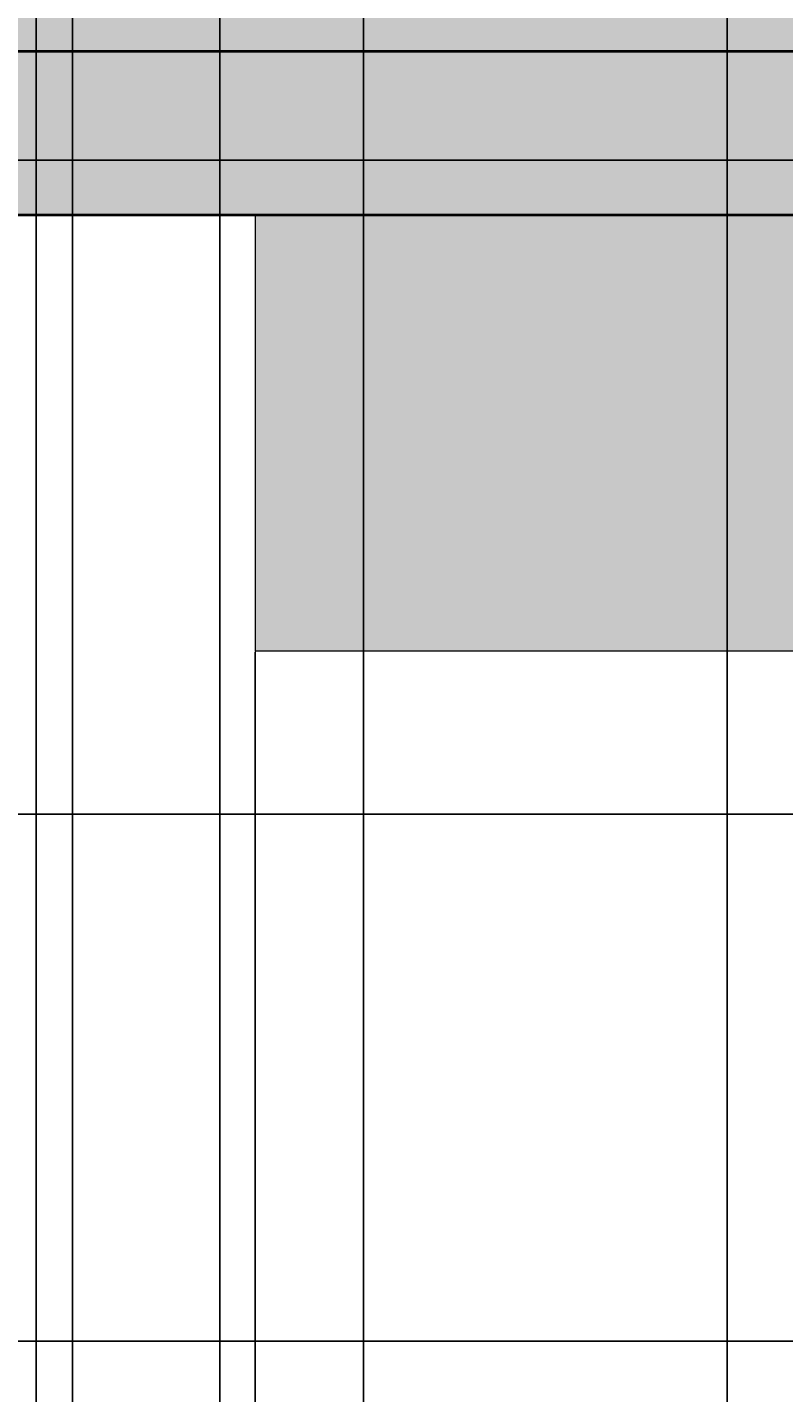
# Model space of a CAD drawing. Units: inches. Extents: x 818 to 1898, y 976 to 2364.
# Tile 84 of 96: x 1439 to 1481, y 1979 to 2054. Entities that reach past the tile are written whole.
import ezdxf

# ---------------------------------------------------------------- set-up
doc = ezdxf.new("R2010")
doc.units = ezdxf.units.IN
doc.header["$LTSCALE"] = 5
doc.header["$MEASUREMENT"] = 0
for name, color, linetype, lineweight in [('A-ANNO-DIMS', 2, 'Continuous', 18), ('A-FLOR-CASE', 8, 'Continuous', 18), ('A-FURN-PATT', 8, 'Continuous', 9), ('A-WALL', 7, 'Continuous', 40)]:
    doc.layers.add(name, color=color, linetype=linetype, lineweight=lineweight)
doc.layers.add('A-WALL-PATT', color=251, linetype='Continuous', lineweight=13, true_color=0x636466)
doc.layers.add('L-PLNT-PATT', color=114, linetype='Continuous', lineweight=9, true_color=0x139b48)
doc.styles.get("Standard").update_dxf_attribs({"font": 'arial.ttf'})
doc.dimstyles.get("Standard").update_dxf_attribs({"dimtxt": 0.18, "dimasz": 0.18, "dimexe": 0.18, "dimexo": 0.0625, "dimgap": 0.09, "dimtad": 0, "dimtih": 1, "dimtoh": 1, "dimdec": 4, "dimzin": 0, "dimdsep": 46, "dimtxsty": 'Standard', "dimcen": 0.09, "dimadec": 0, "dimazin": 0, "dimtfac": 1, "dimtdec": 4, "dimtofl": 0, "dimtmove": 0, "dimatfit": 3, "dimfxl": 1, "dimtolj": 1, "dimtzin": 0, "dimarcsym": 0})

# ---------------------------------------------------------------- blocks, each defined once
blk = doc.blocks.new('*D73')
at = {"layer": 'A-ANNO-DIMS', "color": 0, "lineweight": -2, "ltscale": 5, "transparency": 16777216}
for p, q in [((1590.663, 2011.078), (818.026, 2011.078)), ((818.206, 2010.898), (818.206, 1996.76)), ((818.206, 1982.258), (818.206, 1996.396)), ((1590.663, 1982.078), (818.026, 1982.078))]:
    blk.add_line(p, q, dxfattribs=at)
at = {"layer": 'A-ANNO-DIMS', "color": 0, "ltscale": 5, "transparency": 16777216}
for points in [[(818.176, 2010.898), (818.236, 2010.898), (818.206, 2011.078)], [(818.176, 1982.258), (818.236, 1982.258), (818.206, 1982.078)]]:
    blk.add_solid(points, dxfattribs=at)
at = {"layer": 'Defpoints', "color": 0, "ltscale": 5, "transparency": 16777216}
for p in [(818.206, 2011.078), (1590.725, 2011.078), (1590.725, 1982.078)]:
    blk.add_point(p, dxfattribs=at)
at = {"layer": 'A-ANNO-DIMS', "color": 0, "ltscale": 5, "transparency": 16777216, "insert": (818.206, 1996.578), "char_height": 0.18, "attachment_point": 5}
blk.add_mtext('\\A1;29', dxfattribs=at)
blk = doc.blocks.new('*D85')
at = {"layer": 'A-ANNO-DIMS', "color": 0, "lineweight": -2, "ltscale": 5, "transparency": 16777216}
for p, q in [((1258.788, 2053.078), (1897.916, 2053.078)), ((1897.736, 2052.898), (1897.736, 1876.76)), ((1897.736, 1700.258), (1897.736, 1876.396)), ((1258.788, 1700.078), (1897.916, 1700.078))]:
    blk.add_line(p, q, dxfattribs=at)
at = {"layer": 'A-ANNO-DIMS', "color": 0, "ltscale": 5, "transparency": 16777216}
for points in [[(1897.706, 2052.898), (1897.766, 2052.898), (1897.736, 2053.078)], [(1897.706, 1700.258), (1897.766, 1700.258), (1897.736, 1700.078)]]:
    blk.add_solid(points, dxfattribs=at)
at = {"layer": 'Defpoints', "color": 0, "ltscale": 5, "transparency": 16777216}
for p in [(1258.725, 2053.078), (1897.736, 2053.078), (1258.725, 1700.078)]:
    blk.add_point(p, dxfattribs=at)
at = {"layer": 'A-ANNO-DIMS', "color": 0, "ltscale": 5, "transparency": 16777216, "insert": (1897.736, 1876.578), "char_height": 0.18, "attachment_point": 5}
blk.add_mtext('\\A1;353', dxfattribs=at)
blk = doc.blocks.new('*D86')
at = {"layer": 'A-ANNO-DIMS', "color": 0, "lineweight": -2, "ltscale": 5, "transparency": 16777216}
for p, q in [((1258.725, 2053.141), (1258.725, 2363.873)), ((1258.905, 2363.693), (1486.433, 2363.693)), ((1714.545, 2363.693), (1487.018, 2363.693)), ((1714.725, 2053.141), (1714.725, 2363.873))]:
    blk.add_line(p, q, dxfattribs=at)
at = {"layer": 'A-ANNO-DIMS', "color": 0, "ltscale": 5, "transparency": 16777216}
for points in [[(1258.905, 2363.723), (1258.905, 2363.663), (1258.725, 2363.693)], [(1714.545, 2363.723), (1714.545, 2363.663), (1714.725, 2363.693)]]:
    blk.add_solid(points, dxfattribs=at)
at = {"layer": 'Defpoints', "color": 0, "ltscale": 5, "transparency": 16777216}
for p in [(1714.725, 2363.693), (1258.725, 2053.078), (1714.725, 2053.078)]:
    blk.add_point(p, dxfattribs=at)
at = {"layer": 'A-ANNO-DIMS', "color": 0, "ltscale": 5, "transparency": 16777216, "insert": (1486.725, 2363.693), "char_height": 0.18, "attachment_point": 5}
blk.add_mtext('\\A1;456', dxfattribs=at)
blk = doc.blocks.new('*D99')
at = {"layer": 'A-ANNO-DIMS', "color": 0, "lineweight": -2, "ltscale": 5, "transparency": 16777216}
for p, q in [((1391.876, 1071.118), (1391.876, 2363.873)), ((1392.056, 2363.693), (1420.454, 2363.693)), ((1449.64, 2363.693), (1421.241, 2363.693)), ((1449.82, 1071.118), (1449.82, 2363.873))]:
    blk.add_line(p, q, dxfattribs=at)
at = {"layer": 'A-ANNO-DIMS', "color": 0, "ltscale": 5, "transparency": 16777216}
for points in [[(1392.056, 2363.723), (1392.056, 2363.663), (1391.876, 2363.693)], [(1449.64, 2363.723), (1449.64, 2363.663), (1449.82, 2363.693)]]:
    blk.add_solid(points, dxfattribs=at)
at = {"layer": 'Defpoints', "color": 0, "ltscale": 5, "transparency": 16777216}
for p in [(1449.82, 2363.693), (1391.876, 1071.055), (1449.82, 1071.055)]:
    blk.add_point(p, dxfattribs=at)
at = {"layer": 'A-ANNO-DIMS', "color": 0, "ltscale": 5, "transparency": 16777216, "insert": (1420.848, 2363.693), "char_height": 0.18, "attachment_point": 5}
blk.add_mtext('\\A1;57.94', dxfattribs=at)
blk = doc.blocks.new('*D100')
at = {"layer": 'A-ANNO-DIMS', "color": 0, "lineweight": -2, "ltscale": 5, "transparency": 16777216}
for p, q in [((1449.82, 1071.118), (1449.82, 2363.873)), ((1450, 2363.693), (1478.165, 2363.693)), ((1507.118, 2363.693), (1478.953, 2363.693)), ((1507.298, 1071.118), (1507.298, 2363.873))]:
    blk.add_line(p, q, dxfattribs=at)
at = {"layer": 'A-ANNO-DIMS', "color": 0, "ltscale": 5, "transparency": 16777216}
for points in [[(1450, 2363.723), (1450, 2363.663), (1449.82, 2363.693)], [(1507.118, 2363.723), (1507.118, 2363.663), (1507.298, 2363.693)]]:
    blk.add_solid(points, dxfattribs=at)
at = {"layer": 'Defpoints', "color": 0, "ltscale": 5, "transparency": 16777216}
for p in [(1507.298, 2363.693), (1449.82, 1071.055), (1507.298, 1071.055)]:
    blk.add_point(p, dxfattribs=at)
at = {"layer": 'A-ANNO-DIMS', "color": 0, "ltscale": 5, "transparency": 16777216, "insert": (1478.559, 2363.693), "char_height": 0.18, "attachment_point": 5}
blk.add_mtext('\\A1;57.48', dxfattribs=at)
blk = doc.blocks.new('*D161')
at = {"layer": 'A-ANNO-DIMS', "color": 0, "lineweight": -2, "ltscale": 5, "transparency": 16777216}
for p, q in [((1429.225, 1876.141), (1429.225, 2363.873)), ((1429.405, 2363.693), (1509.589, 2363.693)), ((1590.545, 2363.693), (1510.361, 2363.693)), ((1590.725, 1876.141), (1590.725, 2363.873))]:
    blk.add_line(p, q, dxfattribs=at)
at = {"layer": 'A-ANNO-DIMS', "color": 0, "ltscale": 5, "transparency": 16777216}
for points in [[(1429.405, 2363.723), (1429.405, 2363.663), (1429.225, 2363.693)], [(1590.545, 2363.723), (1590.545, 2363.663), (1590.725, 2363.693)]]:
    blk.add_solid(points, dxfattribs=at)
at = {"layer": 'Defpoints', "color": 0, "ltscale": 5, "transparency": 16777216}
for p in [(1590.725, 2363.693), (1429.225, 1876.078), (1590.725, 1876.078)]:
    blk.add_point(p, dxfattribs=at)
at = {"layer": 'A-ANNO-DIMS', "color": 0, "ltscale": 5, "transparency": 16777216, "insert": (1509.975, 2363.693), "char_height": 0.18, "attachment_point": 5}
blk.add_mtext('\\A1;161.5', dxfattribs=at)
blk = doc.blocks.new('*D169')
at = {"layer": 'A-ANNO-DIMS', "color": 0, "lineweight": -2, "ltscale": 5, "transparency": 16777216}
for p, q in [((1441.725, 1600.141), (1441.725, 2363.873)), ((1441.905, 2363.693), (1459.506, 2363.693)), ((1477.545, 2363.693), (1459.944, 2363.693)), ((1477.725, 1600.141), (1477.725, 2363.873))]:
    blk.add_line(p, q, dxfattribs=at)
at = {"layer": 'A-ANNO-DIMS', "color": 0, "ltscale": 5, "transparency": 16777216}
for points in [[(1441.905, 2363.723), (1441.905, 2363.663), (1441.725, 2363.693)], [(1477.545, 2363.723), (1477.545, 2363.663), (1477.725, 2363.693)]]:
    blk.add_solid(points, dxfattribs=at)
at = {"layer": 'Defpoints', "color": 0, "ltscale": 5, "transparency": 16777216}
for p in [(1477.725, 2363.693), (1441.725, 1600.078), (1477.725, 1600.078)]:
    blk.add_point(p, dxfattribs=at)
at = {"layer": 'A-ANNO-DIMS', "color": 0, "ltscale": 5, "transparency": 16777216, "insert": (1459.725, 2363.693), "char_height": 0.18, "attachment_point": 5}
blk.add_mtext('\\A1;36', dxfattribs=at)
blk = doc.blocks.new('*D196')
at = {"layer": 'A-ANNO-DIMS', "color": 0, "lineweight": -2, "ltscale": 5, "transparency": 16777216}
for p, q in [((1439.725, 1526.734), (1439.725, 2363.873)), ((1439.905, 2363.693), (1448.515, 2363.693)), ((1457.545, 2363.693), (1448.936, 2363.693)), ((1457.725, 1526.734), (1457.725, 2363.873))]:
    blk.add_line(p, q, dxfattribs=at)
at = {"layer": 'A-ANNO-DIMS', "color": 0, "ltscale": 5, "transparency": 16777216}
for points in [[(1439.905, 2363.723), (1439.905, 2363.663), (1439.725, 2363.693)], [(1457.545, 2363.723), (1457.545, 2363.663), (1457.725, 2363.693)]]:
    blk.add_solid(points, dxfattribs=at)
at = {"layer": 'Defpoints', "color": 0, "ltscale": 5, "transparency": 16777216}
for p in [(1457.725, 2363.693), (1439.725, 1526.671), (1457.725, 1526.671)]:
    blk.add_point(p, dxfattribs=at)
at = {"layer": 'A-ANNO-DIMS', "color": 0, "ltscale": 5, "transparency": 16777216, "insert": (1448.725, 2363.693), "char_height": 0.18, "attachment_point": 5}
blk.add_mtext('\\A1;18', dxfattribs=at)
blk = doc.blocks.new('*D207')
at = {"layer": 'A-ANNO-DIMS', "color": 0, "lineweight": -2, "ltscale": 5, "transparency": 16777216}
for p, q in [((1590.663, 2044.078), (818.026, 2044.078)), ((818.206, 2043.898), (818.206, 2027.76)), ((818.206, 2011.258), (818.206, 2027.396)), ((1590.663, 2011.078), (818.026, 2011.078))]:
    blk.add_line(p, q, dxfattribs=at)
at = {"layer": 'A-ANNO-DIMS', "color": 0, "ltscale": 5, "transparency": 16777216}
for points in [[(818.176, 2043.898), (818.236, 2043.898), (818.206, 2044.078)], [(818.176, 2011.258), (818.236, 2011.258), (818.206, 2011.078)]]:
    blk.add_solid(points, dxfattribs=at)
at = {"layer": 'Defpoints', "color": 0, "ltscale": 5, "transparency": 16777216}
for p in [(818.206, 2044.078), (1590.725, 2044.078), (1590.725, 2011.078)]:
    blk.add_point(p, dxfattribs=at)
at = {"layer": 'A-ANNO-DIMS', "color": 0, "ltscale": 5, "transparency": 16777216, "insert": (818.206, 2027.578), "char_height": 0.18, "attachment_point": 5}
blk.add_mtext('\\A1;33', dxfattribs=at)
blk = doc.blocks.new('*D243')
at = {"layer": 'A-ANNO-DIMS', "color": 0, "lineweight": -2, "ltscale": 5, "transparency": 16777216}
for p, q in [((1451.77, 2020.016), (1451.77, 975.663)), ((1590.725, 2020.016), (1590.725, 975.663)), ((1451.95, 975.843), (1520.792, 975.843)), ((1590.545, 975.843), (1521.703, 975.843))]:
    blk.add_line(p, q, dxfattribs=at)
at = {"layer": 'A-ANNO-DIMS', "color": 0, "ltscale": 5, "transparency": 16777216}
for points in [[(1451.95, 975.873), (1451.95, 975.813), (1451.77, 975.843)], [(1590.545, 975.873), (1590.545, 975.813), (1590.725, 975.843)]]:
    blk.add_solid(points, dxfattribs=at)
at = {"layer": 'Defpoints', "color": 0, "ltscale": 5, "transparency": 16777216}
for p in [(1451.77, 2020.078), (1590.725, 2020.078), (1590.725, 975.843)]:
    blk.add_point(p, dxfattribs=at)
at = {"layer": 'A-ANNO-DIMS', "color": 0, "ltscale": 5, "transparency": 16777216, "insert": (1521.247, 975.843), "char_height": 0.18, "attachment_point": 5}
blk.add_mtext('\\A1;138.96', dxfattribs=at)
blk = doc.blocks.new('*D258')
at = {"layer": 'A-ANNO-DIMS', "color": 0, "lineweight": -2, "ltscale": 5, "transparency": 16777216}
for p, q in [((1422.02, 2053.141), (1422.02, 2363.873)), ((1422.2, 2363.693), (1453.264, 2363.693)), ((1484.942, 2363.693), (1453.878, 2363.693)), ((1485.122, 2053.141), (1485.122, 2363.873))]:
    blk.add_line(p, q, dxfattribs=at)
at = {"layer": 'A-ANNO-DIMS', "color": 0, "ltscale": 5, "transparency": 16777216}
for points in [[(1422.2, 2363.723), (1422.2, 2363.663), (1422.02, 2363.693)], [(1484.942, 2363.723), (1484.942, 2363.663), (1485.122, 2363.693)]]:
    blk.add_solid(points, dxfattribs=at)
at = {"layer": 'Defpoints', "color": 0, "ltscale": 5, "transparency": 16777216}
for p in [(1485.122, 2363.693), (1422.02, 2053.078), (1485.122, 2053.078)]:
    blk.add_point(p, dxfattribs=at)
at = {"layer": 'A-ANNO-DIMS', "color": 0, "ltscale": 5, "transparency": 16777216, "insert": (1453.571, 2363.693), "char_height": 0.18, "attachment_point": 5}
blk.add_mtext('\\A1;63.1', dxfattribs=at)
blk = doc.blocks.new('*D266')
at = {"layer": 'A-ANNO-DIMS', "color": 0, "lineweight": -2, "ltscale": 5, "transparency": 16777216}
for p, q in [((1780.439, 2053.078), (818.026, 2053.078)), ((818.206, 2052.898), (818.206, 2050.26)), ((818.206, 2047.258), (818.206, 2049.896)), ((1780.439, 2047.078), (818.026, 2047.078))]:
    blk.add_line(p, q, dxfattribs=at)
at = {"layer": 'A-ANNO-DIMS', "color": 0, "ltscale": 5, "transparency": 16777216}
for points in [[(818.176, 2052.898), (818.236, 2052.898), (818.206, 2053.078)], [(818.176, 2047.258), (818.236, 2047.258), (818.206, 2047.078)]]:
    blk.add_solid(points, dxfattribs=at)
at = {"layer": 'Defpoints', "color": 0, "ltscale": 5, "transparency": 16777216}
for p in [(1780.502, 2053.078), (818.206, 2047.078), (1780.502, 2047.078)]:
    blk.add_point(p, dxfattribs=at)
at = {"layer": 'A-ANNO-DIMS', "color": 0, "ltscale": 5, "transparency": 16777216, "insert": (818.206, 2050.078), "char_height": 0.18, "attachment_point": 5}
blk.add_mtext('\\A1;6', dxfattribs=at)
blk = doc.blocks.new('*D281')
at = {"layer": 'A-ANNO-DIMS', "color": 0, "lineweight": -2, "ltscale": 5, "transparency": 16777216}
for p, q in [((1250.303, 1913.703), (1250.303, 2363.873)), ((1250.483, 2363.693), (1420.121, 2363.693)), ((1590.545, 2363.693), (1420.907, 2363.693)), ((1590.725, 2011.141), (1590.725, 2363.873))]:
    blk.add_line(p, q, dxfattribs=at)
at = {"layer": 'A-ANNO-DIMS', "color": 0, "ltscale": 5, "transparency": 16777216}
for points in [[(1250.483, 2363.723), (1250.483, 2363.663), (1250.303, 2363.693)], [(1590.545, 2363.723), (1590.545, 2363.663), (1590.725, 2363.693)]]:
    blk.add_solid(points, dxfattribs=at)
at = {"layer": 'Defpoints', "color": 0, "ltscale": 5, "transparency": 16777216}
for p in [(1590.725, 2363.693), (1590.725, 2011.078), (1250.303, 1913.64)]:
    blk.add_point(p, dxfattribs=at)
at = {"layer": 'A-ANNO-DIMS', "color": 0, "ltscale": 5, "transparency": 16777216, "insert": (1420.514, 2363.693), "char_height": 0.18, "attachment_point": 5}
blk.add_mtext('\\A1;340.4', dxfattribs=at)
blk = doc.blocks.new('*D282')
at = {"layer": 'A-ANNO-DIMS', "color": 0, "lineweight": -2, "ltscale": 5, "transparency": 16777216}
for p, q in [((1422.083, 2081.188), (1897.916, 2081.188)), ((1897.736, 2081.008), (1897.736, 1884.315)), ((1897.736, 1687.258), (1897.736, 1883.951)), ((1463.788, 1687.078), (1897.916, 1687.078))]:
    blk.add_line(p, q, dxfattribs=at)
at = {"layer": 'A-ANNO-DIMS', "color": 0, "ltscale": 5, "transparency": 16777216}
for points in [[(1897.706, 2081.008), (1897.766, 2081.008), (1897.736, 2081.188)], [(1897.706, 1687.258), (1897.766, 1687.258), (1897.736, 1687.078)]]:
    blk.add_solid(points, dxfattribs=at)
at = {"layer": 'Defpoints', "color": 0, "ltscale": 5, "transparency": 16777216}
for p in [(1422.02, 2081.188), (1897.736, 2081.188), (1463.725, 1687.078)]:
    blk.add_point(p, dxfattribs=at)
at = {"layer": 'A-ANNO-DIMS', "color": 0, "ltscale": 5, "transparency": 16777216, "insert": (1897.736, 1884.133), "char_height": 0.18, "attachment_point": 5}
blk.add_mtext('\\A1;394.1', dxfattribs=at)
blk = doc.blocks.new('*D288')
at = {"layer": 'A-ANNO-DIMS', "color": 0, "lineweight": -2, "ltscale": 5, "transparency": 16777216}
for p, q in [((1422.876, 1742.674), (1422.876, 2363.873)), ((1423.056, 2363.693), (1466.906, 2363.693)), ((1511.545, 2363.693), (1467.695, 2363.693)), ((1511.725, 1716.108), (1511.725, 2363.873))]:
    blk.add_line(p, q, dxfattribs=at)
at = {"layer": 'A-ANNO-DIMS', "color": 0, "ltscale": 5, "transparency": 16777216}
for points in [[(1423.056, 2363.723), (1423.056, 2363.663), (1422.876, 2363.693)], [(1511.545, 2363.723), (1511.545, 2363.663), (1511.725, 2363.693)]]:
    blk.add_solid(points, dxfattribs=at)
at = {"layer": 'Defpoints', "color": 0, "ltscale": 5, "transparency": 16777216}
for p in [(1511.725, 2363.693), (1422.876, 1742.611), (1511.725, 1716.045)]:
    blk.add_point(p, dxfattribs=at)
at = {"layer": 'A-ANNO-DIMS', "color": 0, "ltscale": 5, "transparency": 16777216, "insert": (1467.3, 2363.693), "char_height": 0.18, "attachment_point": 5}
blk.add_mtext('\\A1;88.85', dxfattribs=at)

msp = doc.modelspace()

# ---------------------------------------------------------------- hatches: boundary and pattern name
at = {"layer": 'A-FURN-PATT', "ltscale": 5}
h = msp.add_hatch(color=256, dxfattribs=at)
h.dxf.hatch_style = 1
h.paths.add_polyline_path([(1341.9997, 1981.5338), (1317.9034, 2001.8247), (1314.2595, 2001.8247), (1314.2595, 2004.893), (1310.1046, 2008.3917), (1303.9314, 2008.3917), (1303.9314, 1953.0408), (1308.1629, 1953.0408), (1314.2595, 1958.1746), (1314.2595, 1959.6079), (1315.9616, 1959.6079)])
h.paths.add_polyline_path([(1341.9997, 1981.5338), (1315.9616, 1959.6079), (1336.7936, 1959.6079), (1336.7936, 1953.0408), (1345.3966, 1953.0408), (1345.3966, 1959.6079), (1368.0379, 1959.6079)])
h.paths.add_polyline_path([(1402.518, 2008.3917), (1398.8475, 2008.3917), (1398.8475, 2001.8247), (1376.3134, 2001.8247), (1376.3134, 2008.3917), (1373.8948, 2008.3917), (1367.9307, 2003.3695), (1367.9307, 2001.8247), (1366.0961, 2001.8247), (1341.9997, 1981.5338), (1368.0379, 1959.6079), (1375.8366, 1953.0408), (1376.3134, 1953.0408), (1376.3134, 1959.6079), (1398.8475, 1959.6079), (1398.8475, 1953.0408), (1402.518, 1953.0408)])
h.paths.add_polyline_path([(1366.0961, 2001.8247), (1345.3966, 2001.8247), (1345.3966, 2008.3917), (1336.7936, 2008.3917), (1336.7936, 2001.8247), (1317.9034, 2001.8247), (1341.9997, 1981.5338)])
h.paths.add_polyline_path([(1336.7936, 1959.6079), (1315.9616, 1959.6079), (1314.2595, 1958.1746), (1314.2595, 1953.0408), (1336.7936, 1953.0408)], flags=17)
h.paths.add_polyline_path([(1367.9307, 1959.6079), (1345.3966, 1959.6079), (1345.3966, 1953.0408), (1367.9307, 1953.0408)], flags=17)
h.paths.add_polyline_path([(1398.8475, 1959.6079), (1376.3134, 1959.6079), (1376.3134, 1953.0408), (1398.8475, 1953.0408)], flags=17)
h.paths.add_polyline_path([(1368.0379, 1959.6079), (1367.9307, 1959.6079), (1367.9307, 1953.0408), (1375.8366, 1953.0408)], flags=17)
h.paths.add_polyline_path([(1314.2595, 1958.1746), (1308.1629, 1953.0408), (1314.2595, 1953.0408)], flags=17)
h.paths.add_polyline_path([(1315.9616, 1959.6079), (1314.2595, 1959.6079), (1314.2595, 1958.1746)], flags=16)
h.paths.add_polyline_path([(1314.2595, 2008.3917), (1310.1046, 2008.3917), (1314.2595, 2004.893)], flags=17)
h.paths.add_polyline_path([(1336.7936, 2008.3917), (1314.2595, 2008.3917), (1314.2595, 2004.893), (1317.9034, 2001.8247), (1336.7936, 2001.8247)], flags=17)
h.paths.add_polyline_path([(1314.2595, 2004.893), (1314.2595, 2001.8247), (1317.9034, 2001.8247)], flags=16)
h.paths.add_polyline_path([(1367.9307, 2008.3917), (1345.3966, 2008.3917), (1345.3966, 2001.8247), (1366.0961, 2001.8247), (1367.9307, 2003.3695)], flags=17)
h.paths.add_polyline_path([(1398.8475, 2008.3917), (1376.3134, 2008.3917), (1376.3134, 2001.8247), (1398.8475, 2001.8247)], flags=17)
h.paths.add_polyline_path([(1373.8948, 2008.3917), (1367.9307, 2008.3917), (1367.9307, 2003.3695)], flags=17)
h.paths.add_polyline_path([(1367.9307, 2003.3695), (1366.0961, 2001.8247), (1367.9307, 2001.8247)], flags=16)
h.paths.add_polyline_path([(1546.1595, 2044.0782), (1451.7698, 2044.0782), (1451.7698, 2020.0782), (1546.1595, 2020.0782)])
h.paths.add_polyline_path([(1492.0729, 2040.001, 0.431429), (1491.8238, 2040.251), (1491.3087, 2040.251, 0.415217), (1491.0729, 2040.001)], flags=16)
h.paths.add_polyline_path([(1481.8346, 2039.6036), (1511.886, 2039.6036), (1511.886, 2024.9917), (1481.8346, 2024.9917)], flags=16)
h.paths.add_polyline_path([(1491.0729, 2039.4857), (1491.0729, 2039.501), (1492.0729, 2039.501, -0.4117484), (1491.8401, 2039.251), (1491.8229, 2039.251), (1491.8229, 2039.2509, 0.4325918), (1492.0729, 2039.501), (1491.0729, 2039.501, 0.432604), (1491.3229, 2039.2509), (1491.3229, 2039.251), (1491.325, 2039.251, -0.4165823)], flags=0)
h.paths.add_polyline_path([(1485.3701, 2030.9622), (1485.3701, 2034.3556, -0.4142136), (1488.3701, 2037.3556), (1490.3421, 2037.3556, -0.0779193), (1491.0729, 2038.751), (1495.0729, 2038.751, -0.3148679), (1496.07, 2037.1201, -0.3016609), (1497.9049, 2034.3556), (1497.9049, 2030.9622, -0.4142136), (1494.9049, 2027.9622), (1488.3701, 2027.9622, -0.4142136)], flags=0)
h.paths.add_polyline_path([(1490.3229, 2035.751, 0.2655648), (1491.3229, 2036.751), (1491.3229, 2037.126), (1491.0729, 2037.126, -0.7914183), (1490.5434, 2037.251, -0.7914183), (1491.0729, 2037.376), (1491.3229, 2037.376), (1491.3229, 2037.751), (1492.0729, 2037.751), (1492.0729, 2037.376), (1492.3229, 2037.376, -0.7914183), (1492.8524, 2037.251, -0.7914183), (1492.3229, 2037.126), (1492.1491, 2037.126, -0.0866263), (1492.5376, 2036.0294, 0.1070481), (1493.0729, 2035.751), (1490.3229, 2035.751)], flags=0)
h.paths.add_polyline_path([(1491.9774, 2037.251, -1), (1491.4184, 2037.251, -1)], flags=0)
h.paths.add_polyline_path([(1500.0743, 2028.6045), (1500.0743, 2029.4074), (1510.8414, 2029.4074), (1510.8414, 2028.6045)], flags=0)
h.paths.add_polyline_path([(1500.0743, 2030.5314), (1500.0743, 2031.3342), (1510.8414, 2031.3342), (1510.8414, 2030.5314)], flags=0)
h.paths.add_polyline_path([(1500.0743, 2032.94), (1500.0743, 2033.7428), (1510.8414, 2033.7428), (1510.8414, 2032.94)], flags=0)
h.paths.add_polyline_path([(1500.0743, 2035.7499), (1500.0743, 2036.5528), (1510.8414, 2036.5528), (1510.8414, 2035.7499)], flags=0)
h.paths.add_polyline_path([(1590.7251, 2044.0782), (1576.1595, 2044.0782), (1576.1595, 2020.0782), (1590.7251, 2020.0782)])
h.paths.add_polyline_path([(1668.4429, 2044.0782), (1599.7252, 2044.0782), (1599.7252, 2020.0782), (1668.4429, 2020.0782)])
h.paths.add_polyline_path([(1621.2588, 2040.001, 0.431429), (1621.0097, 2040.251), (1620.4946, 2040.251, 0.415217), (1620.2588, 2040.001)], flags=16)
h.paths.add_polyline_path([(1611.0205, 2024.9917), (1611.0205, 2039.6036), (1641.0719, 2039.6036), (1641.0719, 2024.9917)], flags=16)
h.paths.add_polyline_path([(1620.2588, 2039.4857), (1620.2588, 2039.501), (1621.2588, 2039.501, -0.4117484), (1621.026, 2039.251), (1621.0088, 2039.251), (1621.0088, 2039.2509, 0.4325918), (1621.2588, 2039.501), (1620.2588, 2039.501, 0.432604), (1620.5088, 2039.2509), (1620.5088, 2039.251), (1620.5109, 2039.251, -0.4165823)], flags=0)
h.paths.add_polyline_path([(1614.556, 2030.9622), (1614.556, 2034.3556, -0.4142136), (1617.556, 2037.3556), (1619.528, 2037.3556, -0.0779193), (1620.2588, 2038.751), (1624.2588, 2038.751, -0.3148679), (1625.2559, 2037.1201, -0.3016609), (1627.0908, 2034.3556), (1627.0908, 2030.9622, -0.4142136), (1624.0908, 2027.9622), (1617.556, 2027.9622, -0.4142136)], flags=0)
h.paths.add_polyline_path([(1619.5088, 2035.751, 0.2655648), (1620.5088, 2036.751), (1620.5088, 2037.126), (1620.2588, 2037.126, -0.7914183), (1619.7293, 2037.251, -0.7914183), (1620.2588, 2037.376), (1620.5088, 2037.376), (1620.5088, 2037.751), (1621.2588, 2037.751), (1621.2588, 2037.376), (1621.5088, 2037.376, -0.7914183), (1622.0383, 2037.251, -0.7914183), (1621.5088, 2037.126), (1621.335, 2037.126, -0.0866263), (1621.7235, 2036.0294, 0.1070481), (1622.2588, 2035.751), (1619.5088, 2035.751)], flags=0)
h.paths.add_polyline_path([(1620.6043, 2037.251, -1), (1621.1633, 2037.251, -1)], flags=0)
h.paths.add_polyline_path([(1629.2602, 2028.6045), (1629.2602, 2029.4074), (1640.0273, 2029.4074), (1640.0273, 2028.6045)], flags=0)
h.paths.add_polyline_path([(1629.2602, 2030.5314), (1629.2602, 2031.3342), (1640.0273, 2031.3342), (1640.0273, 2030.5314)], flags=0)
h.paths.add_polyline_path([(1629.2602, 2032.94), (1629.2602, 2033.7428), (1640.0273, 2033.7428), (1640.0273, 2032.94)], flags=0)
h.paths.add_polyline_path([(1629.2602, 2035.7499), (1629.2602, 2036.5528), (1640.0273, 2036.5528), (1640.0273, 2035.7499)], flags=0)
h.paths.add_polyline_path([(1705.7252, 2044.0782), (1698.4429, 2044.0782), (1698.4429, 2020.0782), (1705.7252, 2020.0782)])
h.paths.add_polyline_path([(1705.7252, 1972.0782), (1599.7252, 1972.0782), (1599.7252, 1948.0782), (1705.7252, 1948.0782)])
h.paths.add_polyline_path([(1550.0109, 1979.2444), (1483.5451, 1979.2444), (1483.5451, 1948.6602), (1550.0109, 1948.6602)])
h.paths.add_polyline_path([(1490.2586, 1948.6602), (1488.2586, 1948.6602), (1488.2586, 1941.1742, 0.4142136), (1491.2586, 1938.1742), (1500.7446, 1938.1742, -0.4142136)])
h.paths.add_polyline_path([(1513.2306, 1941.1742), (1513.2306, 1948.6602), (1511.2306, 1948.6602, -0.4142136), (1500.7446, 1938.1742), (1510.2306, 1938.1742, 0.4142136)])
h.paths.add_polyline_path([(1518.778, 1948.6602), (1516.778, 1948.6602), (1516.778, 1941.1742, 0.4142136), (1519.778, 1938.1742), (1529.264, 1938.1742, -0.4142136)])
h.paths.add_polyline_path([(1541.75, 1941.1742), (1541.75, 1948.6602), (1539.75, 1948.6602, -0.4142136), (1529.264, 1938.1742), (1538.75, 1938.1742, 0.4142136)])
h.paths.add_polyline_path([(1590.7251, 1900.0782), (1519.6413, 1900.0782), (1519.6413, 1876.0782), (1590.7251, 1876.0782)])
at = {"layer": 'A-WALL-PATT', "ltscale": 5}
h = msp.add_hatch(color=256, dxfattribs=at)
h.dxf.hatch_style = 1
h.paths.add_polyline_path([(1267.7252, 1928.9218), (1258.7251, 1928.9218), (1258.7251, 1913.6401), (1250.3029, 1913.6401), (1250.3029, 1878.3919), (1258.7251, 1878.3919), (1258.7251, 1862.9652), (1267.7252, 1862.9652)])
h.paths.add_polyline_path([(1267.7252, 1814.9652), (1258.7251, 1814.9652), (1258.7251, 1755.3321), (1267.7252, 1755.3321)])
h.paths.add_polyline_path([(1463.7251, 1696.0782), (1267.7252, 1696.0782), (1267.7252, 1707.3321), (1258.7251, 1707.3321), (1258.7251, 1700.0782), (1251.9333, 1700.0782), (1251.9333, 1687.0782), (1463.7251, 1687.0782)])
h.paths.add_polyline_path([(1714.7251, 1717.3178), (1705.7252, 1717.3178), (1705.7252, 1696.0782), (1599.7252, 1696.0782), (1599.7252, 1790.0782), (1705.7252, 1790.0782), (1705.7252, 1785.6125), (1714.7251, 1785.6125), (1714.7251, 1827.2125), (1705.7252, 1827.2125), (1705.7252, 1802.0782), (1599.7252, 1802.0782), (1599.7252, 1867.0782), (1705.7252, 1867.0782), (1705.7252, 1857.2125), (1714.7251, 1857.2125), (1714.7251, 1930.0316), (1741.8409, 1930.0316), (1741.8409, 1935.0316), (1714.7251, 1935.0316), (1714.7251, 1957.0338), (1741.8409, 1957.0338), (1741.8409, 1962.0338), (1714.7251, 1962.0338), (1705.7252, 1962.0338), (1705.7252, 1948.0782), (1599.7252, 1948.0782), (1599.7252, 1981.0782), (1590.7251, 1981.0782), (1590.7251, 1941.0782), (1620.7252, 1941.0782), (1705.7252, 1941.0782), (1705.7252, 1876.0782), (1599.7252, 1876.0782), (1599.7252, 1911.0782), (1590.7251, 1911.0782), (1590.7251, 1876.0782), (1429.2251, 1876.0782), (1429.2251, 1867.0782), (1511.7251, 1867.0782), (1528.593, 1867.0782), (1595.7252, 1867.0782), (1595.7252, 1773.0782), (1520.7252, 1773.0782), (1520.7252, 1837.5823), (1532.593, 1837.5823), (1532.593, 1867.0782), (1528.593, 1867.0782), (1528.593, 1841.5823), (1511.7251, 1841.5823), (1511.7251, 1744.9714), (1520.7252, 1744.9714), (1520.7252, 1761.0782), (1595.7252, 1761.0782), (1595.7252, 1696.0782), (1520.7252, 1696.0782), (1520.7252, 1716.0454), (1511.7251, 1716.0454), (1511.7251, 1696.0782), (1511.7251, 1687.0782), (1714.7251, 1687.0782)])
h.paths.add_polyline_path([(1714.7251, 2053.0782), (1714.7251, 2081.1881), (1709.7252, 2081.1881), (1709.7252, 2053.0782), (1681.6446, 2053.0782), (1681.6446, 2081.1881), (1676.6446, 2081.1881), (1676.6446, 2053.0782), (1538.5155, 2053.0782), (1538.5155, 2044.0782), (1590.7251, 2044.0782), (1590.7251, 2011.0782), (1599.7252, 2011.0782), (1599.7252, 2044.0782), (1705.7252, 2044.0782), (1705.7252, 2014.5114), (1714.7251, 2014.5114)])
h.paths.add_polyline_path([(1485.1216, 2053.0782), (1422.02, 2053.0782), (1422.02, 2081.1881), (1413.02, 2081.1881), (1413.02, 2053.0782), (1399.6356, 2053.0782), (1399.6356, 2081.1881), (1390.6356, 2081.1881), (1390.6356, 2053.0782), (1388.0315, 2053.0782), (1388.0315, 2044.0782), (1416.2743, 2044.0782), (1485.1216, 2044.0782)])
h.paths.add_polyline_path([(1330.305, 2053.0782), (1258.7251, 2053.0782), (1258.7251, 2019.2871), (1267.7252, 2019.2871), (1267.7252, 2044.0782), (1330.305, 2044.0782)])
h.paths.add_polyline_path([(1258.7251, 2053.0782), (1214.6577, 2053.0782), (1214.6577, 2044.0782), (1258.7251, 2044.0782)])
h.paths.add_polyline_path([(1214.6577, 2053.0782), (1180.349, 2053.0782), (1180.349, 2044.0782), (1214.6577, 2044.0782)])
h.paths.add_polyline_path([(1714.7251, 1639.5782), (1741.8409, 1639.5782), (1741.8409, 1643.5782), (1714.7251, 1643.5782), (1714.7251, 1649.9029), (1705.7252, 1649.9029), (1705.7252, 1600.0782), (1477.7251, 1600.0782), (1477.7251, 1591.0782), (1520.7252, 1591.0782), (1616.7252, 1591.0782), (1616.7252, 1416.6857), (1622.7252, 1416.6857), (1622.7252, 1463.0782), (1624.7252, 1463.0782), (1624.7252, 1467.0782), (1622.7252, 1467.0782), (1622.7252, 1591.0782), (1705.7252, 1591.0782), (1705.7252, 1545.0782), (1714.7251, 1545.0782), (1741.8409, 1545.0782), (1741.8409, 1549.0782), (1714.7251, 1549.0782), (1714.7251, 1593.9175), (1737.8409, 1593.9175), (1737.8409, 1597.9175), (1714.7251, 1597.9175)])
h.paths.add_polyline_path([(1674.9024, 2060.7419), (1714.7045, 2060.7419), (1714.7045, 2073.1061), (1674.9024, 2073.1061)], flags=25)
h.paths.add_polyline_path([(1394.5468, 2061.6618), (1422.2344, 2061.6618), (1422.2344, 2074.0261), (1394.5468, 2074.0261)], flags=24)
at = {"layer": 'L-PLNT-PATT', "ltscale": 5}
h = msp.add_hatch(color=256, dxfattribs=at)
h.dxf.hatch_style = 1
h.paths.add_polyline_path([(1789.7173, 2205.9709), (1083.7252, 2205.9709), (1083.7252, 2083.2623), (1218.1114, 2083.2623), (1218.1114, 2053.0782), (1390.6356, 2053.0782), (1390.6356, 2081.1881), (1399.6356, 2081.1881), (1413.02, 2081.1881), (1422.02, 2081.1881), (1422.02, 2053.0782), (1676.6446, 2053.0782), (1676.6446, 2081.1881), (1714.7251, 2081.1881), (1714.7251, 2081.6235), (1789.7173, 2081.6235)])
h.paths.add_polyline_path([(1388.6037, 2145.2461), (1388.6037, 2122.3767), (1373.4756, 2122.3767), (1373.4756, 2145.2461)], flags=16)
h.paths.add_polyline_path([(1408.6922, 2145.2461), (1423.8203, 2145.2461), (1423.8203, 2122.3767), (1408.6922, 2122.3767)], flags=16)
h.paths.add_polyline_path([(1353.3871, 2155.7839), (1353.3871, 2122.3767), (1338.259, 2122.3767), (1338.259, 2155.7839)], flags=16)
h.paths.add_polyline_path([(1443.9089, 2158.4222), (1459.037, 2158.4222), (1459.037, 2122.3767), (1443.9089, 2122.3767)], flags=16)
h.paths.add_polyline_path([(1318.1705, 2145.2461), (1318.1705, 2122.3767), (1303.0424, 2122.3767), (1303.0424, 2145.2461)], flags=16)
h.paths.add_polyline_path([(1479.1255, 2145.2461), (1494.2536, 2145.2461), (1494.2536, 2122.3767), (1479.1255, 2122.3767)], flags=16)
h.paths.add_polyline_path([(1282.9539, 2145.2461), (1282.9539, 2122.3767), (1267.8258, 2122.3767), (1267.8258, 2145.2461)], flags=16)
h.paths.add_polyline_path([(1514.3421, 2145.2461), (1529.4702, 2145.2461), (1529.4702, 2122.3767), (1514.3421, 2122.3767)], flags=16)
h.paths.add_polyline_path([(1247.7373, 2159.4296), (1247.7373, 2122.3767), (1232.6091, 2122.3767), (1232.6091, 2159.4296)], flags=16)
h.paths.add_polyline_path([(1549.5587, 2156.9246), (1564.6868, 2156.9246), (1564.6868, 2122.3767), (1549.5587, 2122.3767)], flags=16)
h.paths.add_polyline_path([(1212.5206, 2145.2461), (1212.5206, 2122.3767), (1197.3925, 2122.3767), (1197.3925, 2145.2461)], flags=16)
h.paths.add_polyline_path([(1584.7753, 2145.2461), (1599.9034, 2145.2461), (1599.9034, 2122.3767), (1584.7753, 2122.3767)], flags=16)
h.paths.add_polyline_path([(1185.1073, 2104.7786), (1190.6407, 2104.7786), (1185.1073, 2098.2505), (1179.5738, 2104.7786)], flags=16)
h.paths.add_polyline_path([(1619.9919, 2145.2461), (1635.1201, 2145.2461), (1635.1201, 2122.3767), (1619.9919, 2122.3767)], flags=16)
h.paths.add_polyline_path([(1655.2086, 2156.1761), (1670.3367, 2156.1761), (1670.3367, 2122.3767), (1655.2086, 2122.3767)], flags=16)
h.paths.add_polyline_path([(1686.5992, 2145.2461), (1701.7273, 2145.2461), (1701.7273, 2122.3767), (1686.5992, 2122.3767)], flags=16)
h.paths.add_polyline_path([(1715.7616, 2145.2461), (1730.8897, 2145.2461), (1730.8897, 2122.3767), (1715.7616, 2122.3767)], flags=16)
h.paths.add_polyline_path([(1753.1652, 2145.2461), (1776.3312, 2145.2461), (1776.3312, 2115.6891), (1753.1652, 2115.6891)], flags=16)
h.paths.add_polyline_path([(1191.4331, 2146.5159), (1176.7891, 2146.5159), (1176.7891, 2134.1516), (1191.4331, 2134.1516)], flags=24)

# ---------------------------------------------------------------- linework, layer by layer
at = {"layer": 'A-FLOR-CASE'}
for p, q in [((1451.7698, 2044.0782), (1451.7698, 2020.0782)), ((1451.7698, 2020.0782), (1590.7251, 2020.0782))]:
    msp.add_line(p, q, dxfattribs=at)
at = {"layer": 'A-WALL'}
for p, q in [((1422.02, 2053.0782), (1676.6446, 2053.0782)), ((1267.7252, 2044.0782), (1590.7251, 2044.0782))]:
    msp.add_line(p, q, dxfattribs=at)

# ---------------------------------------------------------------- dimensions: what is measured, and where the dimension line sits
at = {"layer": 'A-ANNO-DIMS', "ltscale": 5}
for base, p1, p2, override, picture, middle in [((1590.7251, 2363.6929), (1250.3029, 1913.6401), (1590.7251, 2011.0782), {"dimdec": 1, "dimlfac": 1, "dimrnd": 0, "dimzin": 0, "dimdsep": 46, "dimlunit": 2}, '*D281', (1420.514, 2363.6929)), ((1714.7251, 2363.6929), (1258.7251, 2053.0782), (1714.7251, 2053.0782), {"dimdec": 0, "dimlfac": 1, "dimrnd": 0, "dimzin": 0, "dimdsep": 46, "dimlunit": 2}, '*D86', (1486.7251, 2363.6929)), ((1449.8196, 2363.6929), (1391.8757, 1071.0552), (1449.8196, 1071.0552), {"dimdec": 2, "dimlfac": 1, "dimrnd": 0, "dimzin": 0, "dimdsep": 46, "dimlunit": 2}, '*D99', (1420.8477, 2363.6929)), ((1485.1216, 2363.6929), (1422.02, 2053.0782), (1485.1216, 2053.0782), {"dimdec": 1, "dimlfac": 1, "dimrnd": 0, "dimzin": 0, "dimdsep": 46, "dimlunit": 2}, '*D258', (1453.5708, 2363.6929)), ((1511.7251, 2363.6929), (1422.8756, 1742.6113), (1511.7251, 1716.0454), {"dimdec": 2, "dimlfac": 1, "dimrnd": 0, "dimzin": 0, "dimdsep": 46, "dimlunit": 2}, '*D288', (1467.3004, 2363.6929)), ((1590.7251, 2363.6929), (1429.2251, 1876.0782), (1590.7251, 1876.0782), {"dimdec": 1, "dimlfac": 1, "dimrnd": 0, "dimzin": 0, "dimdsep": 46, "dimlunit": 2}, '*D161', (1509.9751, 2363.6929)), ((1457.7251, 2363.6929), (1439.7251, 1526.6712), (1457.7251, 1526.6712), {"dimdec": 0, "dimlfac": 1, "dimrnd": 0, "dimzin": 0, "dimdsep": 46, "dimlunit": 2}, '*D196', (1448.7251, 2363.6929)), ((1477.7251, 2363.6929), (1441.7251, 1600.0782), (1477.7251, 1600.0782), {"dimdec": 0, "dimlfac": 1, "dimrnd": 0, "dimzin": 0, "dimdsep": 46, "dimlunit": 2}, '*D169', (1459.7251, 2363.6929)), ((1507.2982, 2363.6929), (1449.8196, 1071.0552), (1507.2982, 1071.0552), {"dimdec": 2, "dimlfac": 1, "dimrnd": 0, "dimzin": 0, "dimdsep": 46, "dimlunit": 2}, '*D100', (1478.5589, 2363.6929)), ((1590.7251, 975.8433), (1451.7698, 2020.0782), (1590.7251, 2020.0782), {"dimdec": 2, "dimlfac": 1, "dimrnd": 0, "dimzin": 0, "dimdsep": 46, "dimlunit": 2}, '*D243', (1521.2475, 975.8433))]:
    dim = msp.add_linear_dim(base=base, p1=p1, p2=p2, dimstyle='Standard', override=override, dxfattribs=at)
    dim.commit()
    dim.dimension.update_dxf_attribs({"geometry": picture, "text_midpoint": middle})
for base, p1, p2, override, picture, middle in [((1897.736, 2081.1881), (1463.7251, 1687.0782), (1422.02, 2081.1881), {"dimdec": 1, "dimlfac": 1, "dimrnd": 0, "dimzin": 0, "dimdsep": 46, "dimlunit": 2}, '*D282', (1897.736, 1884.1332)), ((818.2059, 2047.0782), (1780.5019, 2053.0782), (1780.5019, 2047.0782), {"dimdec": 0, "dimlfac": 1, "dimrnd": 0, "dimzin": 0, "dimdsep": 46, "dimlunit": 2}, '*D266', (818.2059, 2050.0782)), ((1897.736, 2053.0782), (1258.7251, 1700.0782), (1258.7251, 2053.0782), {"dimdec": 0, "dimlfac": 1, "dimrnd": 0, "dimzin": 0, "dimdsep": 46, "dimlunit": 2}, '*D85', (1897.736, 1876.5782)), ((818.2059, 2044.0782), (1590.7251, 2011.0782), (1590.7251, 2044.0782), {"dimdec": 0, "dimlfac": 1, "dimrnd": 0, "dimzin": 0, "dimdsep": 46, "dimlunit": 2}, '*D207', (818.2059, 2027.5782)), ((818.2059, 2011.0782), (1590.7251, 1982.0782), (1590.7251, 2011.0782), {"dimdec": 0, "dimlfac": 1, "dimrnd": 0, "dimzin": 0, "dimdsep": 46, "dimlunit": 2}, '*D73', (818.2059, 1996.5782))]:
    dim = msp.add_linear_dim(base=base, p1=p1, p2=p2, angle=90, dimstyle='Standard', override=override, dxfattribs=at)
    dim.commit()
    dim.dimension.update_dxf_attribs({"geometry": picture, "text_midpoint": middle})

doc.saveas('drawing.dxf')
